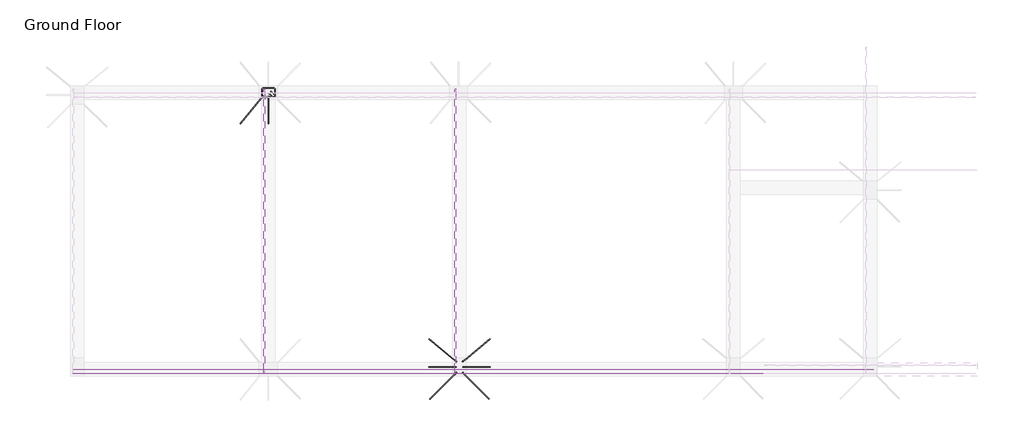
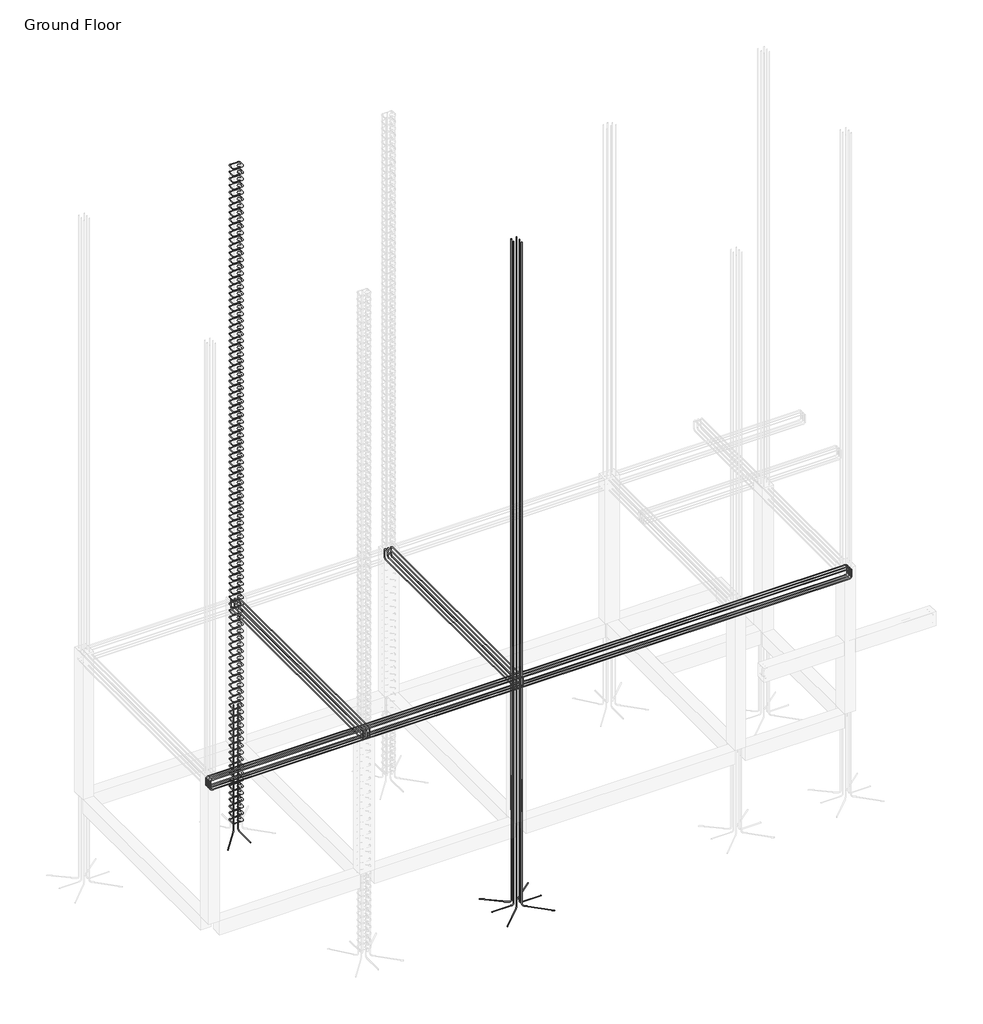
# One storey, part 3 of 5: 21 reinforcing bars.
"""IFC4 building model written with IfcOpenShell, lengths in millimetres."""

from ifc_helpers import new_model, si_unit, point, frame, origin, place, context, project, spatial, polyline, circle_curve, trimmed, segment, composite_curve, source, transform, mapped, element, save
from ifc_brep_helpers import swept_disk

model = new_model("IFC4")

# Units and contexts
model_context = context("Model", 3, world=origin())
ifc_project = project(units=[si_unit("LENGTHUNIT", "METRE", prefix="MILLI")], contexts=[model_context])

# Site, building, storey
site = spatial("IfcSite", under=ifc_project)
building = spatial("IfcBuilding", under=site)
storey = spatial("IfcBuildingStorey", under=building, Name="Ground Floor", Elevation=0.0)

# Reinforcing bars
placement = place(None, origin())
element("IfcReinforcingBar", 1, at=placement, inside=storey, context=model_context, shape_type="SolidModel", body=[
    swept_disk(composite_curve([segment(polyline([(-2783.7729913, 244.7072019, 877.2694454), (-2783.7729913, 244.7072019, -1868.0)]), True, "CONTINUOUS"), segment(trimmed(circle_curve(frame((-2751.2460793, 212.1802899, -1868.0), z_axis=(-0.7071067811865491, -0.707106781186546, 0.0), x_axis=(-32.52691199999981, 32.52691200000001, 0.0)), 46.0), [point((-2783.7729913, 244.7072019, -1868.0))], [point((-2751.2460793, 212.1802899, -1914.0))], True, "CARTESIAN"), True, "CONTINUOUS"), segment(polyline([(-2751.2460793, 212.1802899, -1914.0), (-2345.5428199, -193.5229695, -1914.0)]), True, "CONTINUOUS")], self_intersect=False), 6.0),
])
element("IfcReinforcingBar", 2, at=placement, inside=storey, context=model_context, shape_type="SolidModel", body=[
    swept_disk(composite_curve([segment(polyline([(-2892.5998971, 245.6611074, 884.8983833), (-2892.5998971, 245.6611074, -1868.0)]), True, "CONTINUOUS"), segment(trimmed(circle_curve(frame((-2925.126809, 213.1341954, -1868.0), z_axis=(-0.7071067811865491, 0.707106781186546, 0.0), x_axis=(32.52691189999996, 32.52691199999998, 0.0)), 46.0), [point((-2892.5998971, 245.6611074, -1868.0))], [point((-2925.126809, 213.1341954, -1914.0))], True, "CARTESIAN"), True, "CONTINUOUS"), segment(polyline([(-2925.126809, 213.1341954, -1914.0), (-3337.2563428, -198.9953384, -1914.0)]), True, "CONTINUOUS")], self_intersect=False), 6.0),
])
element("IfcReinforcingBar", 3, at=placement, inside=storey, context=model_context, shape_type="SolidModel", body=[
    swept_disk(composite_curve([segment(polyline([(-2785.0828277, 432.9867911, 871.8711989), (-2785.0828277, 432.9867911, -1868.0)]), True, "CONTINUOUS"), segment(trimmed(circle_curve(frame((-2749.5367573, 462.1839978, -1868.0), z_axis=(0.634721884628903, -0.7727406610067401, 0.0), x_axis=(-35.54607040000019, -29.19720669999998, 0.0)), 46.0), [point((-2785.0828277, 432.9867911, -1868.0))], [point((-2749.5367573, 462.1839978, -1914.0))], True, "CARTESIAN"), True, "CONTINUOUS"), segment(polyline([(-2749.5367573, 462.1839978, -1914.0), (-2327.2008173, 809.0867522, -1914.0)]), True, "CONTINUOUS")], self_intersect=False), 6.0),
])
element("IfcReinforcingBar", 4, at=placement, inside=storey, context=model_context, shape_type="SolidModel", body=[
    swept_disk(composite_curve([segment(polyline([(-2891.7839747, 432.7322479, 890.3940928), (-2891.7839747, 432.7322479, -1868.0)]), True, "CONTINUOUS"), segment(trimmed(circle_curve(frame((-2927.3300451, 461.9294546, -1868.0), z_axis=(0.634721884628903, 0.7727406610067401, 0.0), x_axis=(35.54607040000019, -29.19720669999998, 0.0)), 46.0), [point((-2891.7839747, 432.7322479, -1868.0))], [point((-2927.3300451, 461.9294546, -1914.0))], True, "CARTESIAN"), True, "CONTINUOUS"), segment(polyline([(-2927.3300451, 461.9294546, -1914.0), (-3351.4976875, 810.3367522, -1914.0)]), True, "CONTINUOUS")], self_intersect=False), 6.0),
])
element("IfcReinforcingBar", 5, at=placement, inside=storey, context=model_context, shape_type="SolidModel", body=[
    swept_disk(composite_curve([segment(polyline([(-2778.1117524, 339.6230123, 875.7528218), (-2778.1117524, 339.6230123, -1868.0)]), True, "CONTINUOUS"), segment(trimmed(circle_curve(frame((-2732.1117524, 339.6230123, -1868.0), z_axis=(0.0, -1.0, 0.0), x_axis=(-46.0, 0.0, 0.0)), 46.0), [point((-2778.1117524, 339.6230123, -1868.0))], [point((-2732.1117524, 339.6230123, -1914.0))], True, "CARTESIAN"), True, "CONTINUOUS"), segment(polyline([(-2732.1117524, 339.6230123, -1914.0), (-2321.1359391, 339.6230123, -1914.0)]), True, "CONTINUOUS")], self_intersect=False), 6.0),
])
element("IfcReinforcingBar", 6, at=placement, inside=storey, context=model_context, shape_type="SolidModel", body=[
    swept_disk(composite_curve([segment(polyline([(-2898.7117524, 339.6230123, 879.2840812), (-2898.7117524, 339.6230123, -1868.0)]), True, "CONTINUOUS"), segment(trimmed(circle_curve(frame((-2944.7117524, 339.6230123, -1868.0), z_axis=(0.0, 1.0, 0.0), x_axis=(46.0, 0.0, 0.0)), 46.0), [point((-2898.7117524, 339.6230123, -1868.0))], [point((-2944.7117524, 339.6230123, -1914.0))], True, "CARTESIAN"), True, "CONTINUOUS"), segment(polyline([(-2944.7117524, 339.6230123, -1914.0), (-3358.2222077, 339.6230123, -1914.0)]), True, "CONTINUOUS")], self_intersect=False), 6.0),
])
element("IfcReinforcingBar", 7, at=placement, inside=storey, context=model_context, shape_type="SolidModel", body=[
    swept_disk(composite_curve([segment(polyline([(-2782.2122575, 244.5339681, 12794.2305276), (-2782.2122575, 244.5339681, 171.0746196)]), True, "CONTINUOUS")], self_intersect=False), 6.0),
])
element("IfcReinforcingBar", 8, at=placement, inside=storey, context=model_context, shape_type="SolidModel", body=[
    swept_disk(composite_curve([segment(polyline([(-2778.1117524, 339.6230123, 888.7528218), (-2778.1117524, 339.6230123, 12792.7935546)]), True, "CONTINUOUS")], self_intersect=False), 6.0),
])
element("IfcReinforcingBar", 9, at=placement, inside=storey, context=model_context, shape_type="SolidModel", body=[
    swept_disk(composite_curve([segment(polyline([(-2782.2122575, 433.132958, 12790.6127039), (-2782.2122575, 433.132958, 154.6015232)]), True, "CONTINUOUS")], self_intersect=False), 6.0),
])
element("IfcReinforcingBar", 10, at=placement, inside=storey, context=model_context, shape_type="SolidModel", body=[
    swept_disk(composite_curve([segment(polyline([(-2894.6112474, 244.5339681, 12794.2305276), (-2894.6112474, 244.5339681, 159.2991411)]), True, "CONTINUOUS")], self_intersect=False), 6.0),
])
element("IfcReinforcingBar", 11, at=placement, inside=storey, context=model_context, shape_type="SolidModel", body=[
    swept_disk(composite_curve([segment(polyline([(-2898.7117524, 339.6230123, 892.2840812), (-2898.7117524, 339.6230123, 12792.7935546)]), True, "CONTINUOUS")], self_intersect=False), 6.0),
])
element("IfcReinforcingBar", 12, at=placement, inside=storey, context=model_context, shape_type="SolidModel", body=[
    swept_disk(composite_curve([segment(polyline([(-2894.6112474, 433.132958, 12790.6127039), (-2894.6112474, 433.132958, 134.6074908)]), True, "CONTINUOUS")], self_intersect=False), 6.0),
])
element("IfcReinforcingBar", 13, at=placement, inside=storey, context=model_context, shape_type="SolidModel", body=[
    swept_disk(composite_curve([segment(polyline([(-6145.4105373, 4895.5612408, 890.3940928), (-6145.4105373, 4895.5612408, -1868.0)]), True, "CONTINUOUS"), segment(trimmed(circle_curve(frame((-6174.607744, 4860.0151704, -1868.0), z_axis=(-0.772740661006739, 0.6347218846289044, 0.0), x_axis=(29.197206699999697, 35.546070399999735, 0.0)), 46.0), [point((-6145.4105373, 4895.5612408, -1868.0))], [point((-6174.607744, 4860.0151704, -1914.0))], True, "CARTESIAN"), True, "CONTINUOUS"), segment(polyline([(-6174.607744, 4860.0151704, -1914.0), (-6523.0150416, 4435.8475279, -1914.0)]), True, "CONTINUOUS")], self_intersect=False), 6.0),
])
element("IfcReinforcingBar", 14, at=placement, inside=storey, context=model_context, shape_type="SolidModel", body=[
    swept_disk(composite_curve([segment(polyline([(-6052.3013017, 4888.6334631, 879.2840812), (-6052.3013017, 4888.6334631, -1868.0)]), True, "CONTINUOUS"), segment(trimmed(circle_curve(frame((-6052.3013017, 4842.6334631, -1868.0), z_axis=(-1.0, 0.0, 0.0), x_axis=(0.0, 46.0, 0.0)), 46.0), [point((-6052.3013017, 4888.6334631, -1868.0))], [point((-6052.3013017, 4842.6334631, -1914.0))], True, "CARTESIAN"), True, "CONTINUOUS"), segment(polyline([(-6052.3013017, 4842.6334631, -1914.0), (-6052.3013017, 4429.1230078, -1914.0)]), True, "CONTINUOUS")], self_intersect=False), 6.0),
])
reinforcing_bar_shape = source(origin(), model_context, "Body", "SolidModel", [
    swept_disk(composite_curve([segment(polyline([(-6041.6771046, 4943.2576897, -1724.0), (-5984.0823152, 4885.6629003, -1724.0)]), True, "CONTINUOUS"), segment(trimmed(circle_curve(frame((-5967.1117524, 4902.6334631, -1724.0), z_axis=(0.0, 0.0, 1.0), x_axis=(-16.970562800000152, -16.970562800000152, 0.0)), 24.0), [point((-5984.0823152, 4885.6629003, -1724.0))], [point((-5943.1117524, 4902.6334631, -1724.0))], True, "CARTESIAN"), True, "CONTINUOUS"), segment(polyline([(-5943.1117524, 4902.6334631, -1724.0), (-5943.1117524, 5010.2334631, -1724.0)]), True, "CONTINUOUS"), segment(trimmed(circle_curve(frame((-5967.1117524, 5010.2334631, -1724.0), z_axis=(0.0, 0.0, 1.0), x_axis=(24.0, 0.0, 0.0)), 24.0), [point((-5943.1117524, 5010.2334631, -1724.0))], [point((-5967.1117524, 5034.2334631, -1724.0))], True, "CARTESIAN"), True, "CONTINUOUS"), segment(polyline([(-5967.1117524, 5034.2334631, -1724.0), (-6135.9117524, 5034.2334631, -1724.0)]), True, "CONTINUOUS"), segment(trimmed(circle_curve(frame((-6135.9117524, 5010.2651209, -1725.2323055), z_axis=(0.0, -0.05134606277295722, 0.9986809209340667), x_axis=(0.0, 23.968342200000734, 1.2323054999999385)), 24.0), [point((-6135.9117524, 5034.2334631, -1724.0))], [point((-6159.9117524, 5010.2651209, -1725.2323055))], True, "CARTESIAN"), True, "CONTINUOUS"), segment(polyline([(-6159.9117524, 5010.2651209, -1725.2323055), (-6159.9117524, 4902.6018052, -1730.7676945)]), True, "CONTINUOUS"), segment(trimmed(circle_curve(frame((-6135.9117524, 4902.6018052, -1730.7676945), z_axis=(0.0, -0.05134606277295722, 0.9986809209340667), x_axis=(-24.0, 0.0, 0.0)), 24.0), [point((-6159.9117524, 4902.6018052, -1730.7676945))], [point((-6135.9117524, 4878.6334631, -1732.0))], True, "CARTESIAN"), True, "CONTINUOUS"), segment(polyline([(-6135.9117524, 4878.6334631, -1732.0), (-5967.1117524, 4878.6334631, -1732.0)]), True, "CONTINUOUS"), segment(trimmed(circle_curve(frame((-5967.1117524, 4902.6334631, -1732.0), z_axis=(0.0, 0.0, 1.0), x_axis=(0.0, -24.0, 0.0)), 24.0), [point((-5967.1117524, 4878.6334631, -1732.0))], [point((-5950.1411897, 4919.6040258, -1732.0))], True, "CARTESIAN"), True, "CONTINUOUS"), segment(polyline([(-5950.1411897, 4919.6040258, -1732.0), (-6007.7359791, 4977.1988152, -1732.0)]), True, "CONTINUOUS")], self_intersect=False), 4.0),
])
element("IfcReinforcingBar", 15, at=placement, inside=storey, context=model_context, shape_type="MappedRepresentation", body=[
    mapped(reinforcing_bar_shape, transform((0.0, 0.0, 0.0), x_axis=(1.0, 0.0, 0.0), y_axis=(0.0, 1.0, 0.0), z_axis=(0.0, 0.0, 1.0))),
    mapped(reinforcing_bar_shape, transform((0.0, 0.0, 149.5904239), x_axis=(1.0, 0.0, 0.0), y_axis=(0.0, 1.0, 0.0), z_axis=(0.0, 0.0, 1.0))),
    mapped(reinforcing_bar_shape, transform((0.0, 0.0, 299.1808479), x_axis=(1.0, 0.0, 0.0), y_axis=(0.0, 1.0, 0.0), z_axis=(0.0, 0.0, 1.0))),
    mapped(reinforcing_bar_shape, transform((0.0, 0.0, 448.7712718), x_axis=(1.0, 0.0, 0.0), y_axis=(0.0, 1.0, 0.0), z_axis=(0.0, 0.0, 1.0))),
    mapped(reinforcing_bar_shape, transform((0.0, 0.0, 598.3616957), x_axis=(1.0, 0.0, 0.0), y_axis=(0.0, 1.0, 0.0), z_axis=(0.0, 0.0, 1.0))),
    mapped(reinforcing_bar_shape, transform((0.0, 0.0, 747.9521197), x_axis=(1.0, 0.0, 0.0), y_axis=(0.0, 1.0, 0.0), z_axis=(0.0, 0.0, 1.0))),
    mapped(reinforcing_bar_shape, transform((0.0, 0.0, 897.5425436), x_axis=(1.0, 0.0, 0.0), y_axis=(0.0, 1.0, 0.0), z_axis=(0.0, 0.0, 1.0))),
    mapped(reinforcing_bar_shape, transform((0.0, 0.0, 1047.1329675), x_axis=(1.0, 0.0, 0.0), y_axis=(0.0, 1.0, 0.0), z_axis=(0.0, 0.0, 1.0))),
    mapped(reinforcing_bar_shape, transform((0.0, 0.0, 1196.7233914), x_axis=(1.0, 0.0, 0.0), y_axis=(0.0, 1.0, 0.0), z_axis=(0.0, 0.0, 1.0))),
    mapped(reinforcing_bar_shape, transform((0.0, 0.0, 1346.3138154), x_axis=(1.0, 0.0, 0.0), y_axis=(0.0, 1.0, 0.0), z_axis=(0.0, 0.0, 1.0))),
    mapped(reinforcing_bar_shape, transform((0.0, 0.0, 1495.9042393), x_axis=(1.0, 0.0, 0.0), y_axis=(0.0, 1.0, 0.0), z_axis=(0.0, 0.0, 1.0))),
    mapped(reinforcing_bar_shape, transform((0.0, 0.0, 1645.4946632), x_axis=(1.0, 0.0, 0.0), y_axis=(0.0, 1.0, 0.0), z_axis=(0.0, 0.0, 1.0))),
    mapped(reinforcing_bar_shape, transform((0.0, 0.0, 1795.0850872), x_axis=(1.0, 0.0, 0.0), y_axis=(0.0, 1.0, 0.0), z_axis=(0.0, 0.0, 1.0))),
    mapped(reinforcing_bar_shape, transform((0.0, 0.0, 1944.6755111), x_axis=(1.0, 0.0, 0.0), y_axis=(0.0, 1.0, 0.0), z_axis=(0.0, 0.0, 1.0))),
    mapped(reinforcing_bar_shape, transform((0.0, 0.0, 2094.265935), x_axis=(1.0, 0.0, 0.0), y_axis=(0.0, 1.0, 0.0), z_axis=(0.0, 0.0, 1.0))),
    mapped(reinforcing_bar_shape, transform((0.0, 0.0, 2243.856359), x_axis=(1.0, 0.0, 0.0), y_axis=(0.0, 1.0, 0.0), z_axis=(0.0, 0.0, 1.0))),
    mapped(reinforcing_bar_shape, transform((0.0, 0.0, 2393.4467829), x_axis=(1.0, 0.0, 0.0), y_axis=(0.0, 1.0, 0.0), z_axis=(0.0, 0.0, 1.0))),
    mapped(reinforcing_bar_shape, transform((0.0, 0.0, 2543.0372068), x_axis=(1.0, 0.0, 0.0), y_axis=(0.0, 1.0, 0.0), z_axis=(0.0, 0.0, 1.0))),
    mapped(reinforcing_bar_shape, transform((0.0, 0.0, 2692.6276307), x_axis=(1.0, 0.0, 0.0), y_axis=(0.0, 1.0, 0.0), z_axis=(0.0, 0.0, 1.0))),
    mapped(reinforcing_bar_shape, transform((0.0, 0.0, 2842.2180547), x_axis=(1.0, 0.0, 0.0), y_axis=(0.0, 1.0, 0.0), z_axis=(0.0, 0.0, 1.0))),
    mapped(reinforcing_bar_shape, transform((0.0, 0.0, 2991.8084786), x_axis=(1.0, 0.0, 0.0), y_axis=(0.0, 1.0, 0.0), z_axis=(0.0, 0.0, 1.0))),
    mapped(reinforcing_bar_shape, transform((0.0, 0.0, 3141.3989025), x_axis=(1.0, 0.0, 0.0), y_axis=(0.0, 1.0, 0.0), z_axis=(0.0, 0.0, 1.0))),
    mapped(reinforcing_bar_shape, transform((0.0, 0.0, 3290.9893265), x_axis=(1.0, 0.0, 0.0), y_axis=(0.0, 1.0, 0.0), z_axis=(0.0, 0.0, 1.0))),
    mapped(reinforcing_bar_shape, transform((0.0, 0.0, 3440.5797504), x_axis=(1.0, 0.0, 0.0), y_axis=(0.0, 1.0, 0.0), z_axis=(0.0, 0.0, 1.0))),
    mapped(reinforcing_bar_shape, transform((0.0, 0.0, 3590.1701743), x_axis=(1.0, 0.0, 0.0), y_axis=(0.0, 1.0, 0.0), z_axis=(0.0, 0.0, 1.0))),
    mapped(reinforcing_bar_shape, transform((0.0, 0.0, 3739.7605983), x_axis=(1.0, 0.0, 0.0), y_axis=(0.0, 1.0, 0.0), z_axis=(0.0, 0.0, 1.0))),
    mapped(reinforcing_bar_shape, transform((0.0, 0.0, 3889.3510222), x_axis=(1.0, 0.0, 0.0), y_axis=(0.0, 1.0, 0.0), z_axis=(0.0, 0.0, 1.0))),
    mapped(reinforcing_bar_shape, transform((0.0, 0.0, 4038.9414461), x_axis=(1.0, 0.0, 0.0), y_axis=(0.0, 1.0, 0.0), z_axis=(0.0, 0.0, 1.0))),
    mapped(reinforcing_bar_shape, transform((0.0, 0.0, 4188.53187), x_axis=(1.0, 0.0, 0.0), y_axis=(0.0, 1.0, 0.0), z_axis=(0.0, 0.0, 1.0))),
    mapped(reinforcing_bar_shape, transform((0.0, 0.0, 4338.122294), x_axis=(1.0, 0.0, 0.0), y_axis=(0.0, 1.0, 0.0), z_axis=(0.0, 0.0, 1.0))),
    mapped(reinforcing_bar_shape, transform((0.0, 0.0, 4487.7127179), x_axis=(1.0, 0.0, 0.0), y_axis=(0.0, 1.0, 0.0), z_axis=(0.0, 0.0, 1.0))),
    mapped(reinforcing_bar_shape, transform((0.0, 0.0, 4637.3031418), x_axis=(1.0, 0.0, 0.0), y_axis=(0.0, 1.0, 0.0), z_axis=(0.0, 0.0, 1.0))),
    mapped(reinforcing_bar_shape, transform((0.0, 0.0, 4786.8935658), x_axis=(1.0, 0.0, 0.0), y_axis=(0.0, 1.0, 0.0), z_axis=(0.0, 0.0, 1.0))),
    mapped(reinforcing_bar_shape, transform((0.0, 0.0, 4936.4839897), x_axis=(1.0, 0.0, 0.0), y_axis=(0.0, 1.0, 0.0), z_axis=(0.0, 0.0, 1.0))),
    mapped(reinforcing_bar_shape, transform((0.0, 0.0, 5086.0744136), x_axis=(1.0, 0.0, 0.0), y_axis=(0.0, 1.0, 0.0), z_axis=(0.0, 0.0, 1.0))),
    mapped(reinforcing_bar_shape, transform((0.0, 0.0, 5235.6648376), x_axis=(1.0, 0.0, 0.0), y_axis=(0.0, 1.0, 0.0), z_axis=(0.0, 0.0, 1.0))),
    mapped(reinforcing_bar_shape, transform((0.0, 0.0, 5385.2552615), x_axis=(1.0, 0.0, 0.0), y_axis=(0.0, 1.0, 0.0), z_axis=(0.0, 0.0, 1.0))),
    mapped(reinforcing_bar_shape, transform((0.0, 0.0, 5534.8456854), x_axis=(1.0, 0.0, 0.0), y_axis=(0.0, 1.0, 0.0), z_axis=(0.0, 0.0, 1.0))),
    mapped(reinforcing_bar_shape, transform((0.0, 0.0, 5684.4361094), x_axis=(1.0, 0.0, 0.0), y_axis=(0.0, 1.0, 0.0), z_axis=(0.0, 0.0, 1.0))),
    mapped(reinforcing_bar_shape, transform((0.0, 0.0, 5834.0265333), x_axis=(1.0, 0.0, 0.0), y_axis=(0.0, 1.0, 0.0), z_axis=(0.0, 0.0, 1.0))),
    mapped(reinforcing_bar_shape, transform((0.0, 0.0, 5983.6169572), x_axis=(1.0, 0.0, 0.0), y_axis=(0.0, 1.0, 0.0), z_axis=(0.0, 0.0, 1.0))),
    mapped(reinforcing_bar_shape, transform((0.0, 0.0, 6133.2073811), x_axis=(1.0, 0.0, 0.0), y_axis=(0.0, 1.0, 0.0), z_axis=(0.0, 0.0, 1.0))),
    mapped(reinforcing_bar_shape, transform((0.0, 0.0, 6282.7978051), x_axis=(1.0, 0.0, 0.0), y_axis=(0.0, 1.0, 0.0), z_axis=(0.0, 0.0, 1.0))),
    mapped(reinforcing_bar_shape, transform((0.0, 0.0, 6432.388229), x_axis=(1.0, 0.0, 0.0), y_axis=(0.0, 1.0, 0.0), z_axis=(0.0, 0.0, 1.0))),
    mapped(reinforcing_bar_shape, transform((0.0, 0.0, 6581.9786529), x_axis=(1.0, 0.0, 0.0), y_axis=(0.0, 1.0, 0.0), z_axis=(0.0, 0.0, 1.0))),
    mapped(reinforcing_bar_shape, transform((0.0, 0.0, 6731.5690769), x_axis=(1.0, 0.0, 0.0), y_axis=(0.0, 1.0, 0.0), z_axis=(0.0, 0.0, 1.0))),
    mapped(reinforcing_bar_shape, transform((0.0, 0.0, 6881.1595008), x_axis=(1.0, 0.0, 0.0), y_axis=(0.0, 1.0, 0.0), z_axis=(0.0, 0.0, 1.0))),
    mapped(reinforcing_bar_shape, transform((0.0, 0.0, 7030.7499247), x_axis=(1.0, 0.0, 0.0), y_axis=(0.0, 1.0, 0.0), z_axis=(0.0, 0.0, 1.0))),
    mapped(reinforcing_bar_shape, transform((0.0, 0.0, 7180.3403487), x_axis=(1.0, 0.0, 0.0), y_axis=(0.0, 1.0, 0.0), z_axis=(0.0, 0.0, 1.0))),
    mapped(reinforcing_bar_shape, transform((0.0, 0.0, 7329.9307726), x_axis=(1.0, 0.0, 0.0), y_axis=(0.0, 1.0, 0.0), z_axis=(0.0, 0.0, 1.0))),
    mapped(reinforcing_bar_shape, transform((0.0, 0.0, 7479.5211965), x_axis=(1.0, 0.0, 0.0), y_axis=(0.0, 1.0, 0.0), z_axis=(0.0, 0.0, 1.0))),
    mapped(reinforcing_bar_shape, transform((0.0, 0.0, 7629.1116204), x_axis=(1.0, 0.0, 0.0), y_axis=(0.0, 1.0, 0.0), z_axis=(0.0, 0.0, 1.0))),
    mapped(reinforcing_bar_shape, transform((0.0, 0.0, 7778.7020444), x_axis=(1.0, 0.0, 0.0), y_axis=(0.0, 1.0, 0.0), z_axis=(0.0, 0.0, 1.0))),
    mapped(reinforcing_bar_shape, transform((0.0, 0.0, 7928.2924683), x_axis=(1.0, 0.0, 0.0), y_axis=(0.0, 1.0, 0.0), z_axis=(0.0, 0.0, 1.0))),
    mapped(reinforcing_bar_shape, transform((0.0, 0.0, 8077.8828922), x_axis=(1.0, 0.0, 0.0), y_axis=(0.0, 1.0, 0.0), z_axis=(0.0, 0.0, 1.0))),
    mapped(reinforcing_bar_shape, transform((0.0, 0.0, 8227.4733162), x_axis=(1.0, 0.0, 0.0), y_axis=(0.0, 1.0, 0.0), z_axis=(0.0, 0.0, 1.0))),
    mapped(reinforcing_bar_shape, transform((0.0, 0.0, 8377.0637401), x_axis=(1.0, 0.0, 0.0), y_axis=(0.0, 1.0, 0.0), z_axis=(0.0, 0.0, 1.0))),
    mapped(reinforcing_bar_shape, transform((0.0, 0.0, 8526.654164), x_axis=(1.0, 0.0, 0.0), y_axis=(0.0, 1.0, 0.0), z_axis=(0.0, 0.0, 1.0))),
    mapped(reinforcing_bar_shape, transform((0.0, 0.0, 8676.244588), x_axis=(1.0, 0.0, 0.0), y_axis=(0.0, 1.0, 0.0), z_axis=(0.0, 0.0, 1.0))),
    mapped(reinforcing_bar_shape, transform((0.0, 0.0, 8825.8350119), x_axis=(1.0, 0.0, 0.0), y_axis=(0.0, 1.0, 0.0), z_axis=(0.0, 0.0, 1.0))),
    mapped(reinforcing_bar_shape, transform((0.0, 0.0, 8975.4254358), x_axis=(1.0, 0.0, 0.0), y_axis=(0.0, 1.0, 0.0), z_axis=(0.0, 0.0, 1.0))),
    mapped(reinforcing_bar_shape, transform((0.0, 0.0, 9125.0158597), x_axis=(1.0, 0.0, 0.0), y_axis=(0.0, 1.0, 0.0), z_axis=(0.0, 0.0, 1.0))),
    mapped(reinforcing_bar_shape, transform((0.0, 0.0, 9274.6062837), x_axis=(1.0, 0.0, 0.0), y_axis=(0.0, 1.0, 0.0), z_axis=(0.0, 0.0, 1.0))),
    mapped(reinforcing_bar_shape, transform((0.0, 0.0, 9424.1967076), x_axis=(1.0, 0.0, 0.0), y_axis=(0.0, 1.0, 0.0), z_axis=(0.0, 0.0, 1.0))),
    mapped(reinforcing_bar_shape, transform((0.0, 0.0, 9573.7871315), x_axis=(1.0, 0.0, 0.0), y_axis=(0.0, 1.0, 0.0), z_axis=(0.0, 0.0, 1.0))),
    mapped(reinforcing_bar_shape, transform((0.0, 0.0, 9723.3775555), x_axis=(1.0, 0.0, 0.0), y_axis=(0.0, 1.0, 0.0), z_axis=(0.0, 0.0, 1.0))),
    mapped(reinforcing_bar_shape, transform((0.0, 0.0, 9872.9679794), x_axis=(1.0, 0.0, 0.0), y_axis=(0.0, 1.0, 0.0), z_axis=(0.0, 0.0, 1.0))),
    mapped(reinforcing_bar_shape, transform((0.0, 0.0, 10022.5584033), x_axis=(1.0, 0.0, 0.0), y_axis=(0.0, 1.0, 0.0), z_axis=(0.0, 0.0, 1.0))),
    mapped(reinforcing_bar_shape, transform((0.0, 0.0, 10172.1488273), x_axis=(1.0, 0.0, 0.0), y_axis=(0.0, 1.0, 0.0), z_axis=(0.0, 0.0, 1.0))),
    mapped(reinforcing_bar_shape, transform((0.0, 0.0, 10321.7392512), x_axis=(1.0, 0.0, 0.0), y_axis=(0.0, 1.0, 0.0), z_axis=(0.0, 0.0, 1.0))),
    mapped(reinforcing_bar_shape, transform((0.0, 0.0, 10471.3296751), x_axis=(1.0, 0.0, 0.0), y_axis=(0.0, 1.0, 0.0), z_axis=(0.0, 0.0, 1.0))),
    mapped(reinforcing_bar_shape, transform((0.0, 0.0, 10620.9200991), x_axis=(1.0, 0.0, 0.0), y_axis=(0.0, 1.0, 0.0), z_axis=(0.0, 0.0, 1.0))),
    mapped(reinforcing_bar_shape, transform((0.0, 0.0, 10770.510523), x_axis=(1.0, 0.0, 0.0), y_axis=(0.0, 1.0, 0.0), z_axis=(0.0, 0.0, 1.0))),
    mapped(reinforcing_bar_shape, transform((0.0, 0.0, 10920.1009469), x_axis=(1.0, 0.0, 0.0), y_axis=(0.0, 1.0, 0.0), z_axis=(0.0, 0.0, 1.0))),
    mapped(reinforcing_bar_shape, transform((0.0, 0.0, 11069.6913708), x_axis=(1.0, 0.0, 0.0), y_axis=(0.0, 1.0, 0.0), z_axis=(0.0, 0.0, 1.0))),
    mapped(reinforcing_bar_shape, transform((0.0, 0.0, 11219.2817948), x_axis=(1.0, 0.0, 0.0), y_axis=(0.0, 1.0, 0.0), z_axis=(0.0, 0.0, 1.0))),
    mapped(reinforcing_bar_shape, transform((0.0, 0.0, 11368.8722187), x_axis=(1.0, 0.0, 0.0), y_axis=(0.0, 1.0, 0.0), z_axis=(0.0, 0.0, 1.0))),
    mapped(reinforcing_bar_shape, transform((0.0, 0.0, 11518.4626426), x_axis=(1.0, 0.0, 0.0), y_axis=(0.0, 1.0, 0.0), z_axis=(0.0, 0.0, 1.0))),
    mapped(reinforcing_bar_shape, transform((0.0, 0.0, 11668.0530666), x_axis=(1.0, 0.0, 0.0), y_axis=(0.0, 1.0, 0.0), z_axis=(0.0, 0.0, 1.0))),
    mapped(reinforcing_bar_shape, transform((0.0, 0.0, 11817.6434905), x_axis=(1.0, 0.0, 0.0), y_axis=(0.0, 1.0, 0.0), z_axis=(0.0, 0.0, 1.0))),
    mapped(reinforcing_bar_shape, transform((0.0, 0.0, 11967.2339144), x_axis=(1.0, 0.0, 0.0), y_axis=(0.0, 1.0, 0.0), z_axis=(0.0, 0.0, 1.0))),
    mapped(reinforcing_bar_shape, transform((0.0, 0.0, 12116.8243384), x_axis=(1.0, 0.0, 0.0), y_axis=(0.0, 1.0, 0.0), z_axis=(0.0, 0.0, 1.0))),
    mapped(reinforcing_bar_shape, transform((0.0, 0.0, 12266.4147623), x_axis=(1.0, 0.0, 0.0), y_axis=(0.0, 1.0, 0.0), z_axis=(0.0, 0.0, 1.0))),
    mapped(reinforcing_bar_shape, transform((0.0, 0.0, 12416.0051862), x_axis=(1.0, 0.0, 0.0), y_axis=(0.0, 1.0, 0.0), z_axis=(0.0, 0.0, 1.0))),
    mapped(reinforcing_bar_shape, transform((0.0, 0.0, 12565.5956101), x_axis=(1.0, 0.0, 0.0), y_axis=(0.0, 1.0, 0.0), z_axis=(0.0, 0.0, 1.0))),
    mapped(reinforcing_bar_shape, transform((0.0, 0.0, 12715.1860341), x_axis=(1.0, 0.0, 0.0), y_axis=(0.0, 1.0, 0.0), z_axis=(0.0, 0.0, 1.0))),
    mapped(reinforcing_bar_shape, transform((0.0, 0.0, 12864.776458), x_axis=(1.0, 0.0, 0.0), y_axis=(0.0, 1.0, 0.0), z_axis=(0.0, 0.0, 1.0))),
    mapped(reinforcing_bar_shape, transform((0.0, 0.0, 13014.3668819), x_axis=(1.0, 0.0, 0.0), y_axis=(0.0, 1.0, 0.0), z_axis=(0.0, 0.0, 1.0))),
    mapped(reinforcing_bar_shape, transform((0.0, 0.0, 13163.9573059), x_axis=(1.0, 0.0, 0.0), y_axis=(0.0, 1.0, 0.0), z_axis=(0.0, 0.0, 1.0))),
    mapped(reinforcing_bar_shape, transform((0.0, 0.0, 13313.5477298), x_axis=(1.0, 0.0, 0.0), y_axis=(0.0, 1.0, 0.0), z_axis=(0.0, 0.0, 1.0))),
    mapped(reinforcing_bar_shape, transform((0.0, 0.0, 13463.1381537), x_axis=(1.0, 0.0, 0.0), y_axis=(0.0, 1.0, 0.0), z_axis=(0.0, 0.0, 1.0))),
    mapped(reinforcing_bar_shape, transform((0.0, 0.0, 13612.7285777), x_axis=(1.0, 0.0, 0.0), y_axis=(0.0, 1.0, 0.0), z_axis=(0.0, 0.0, 1.0))),
    mapped(reinforcing_bar_shape, transform((0.0, 0.0, 13762.3190016), x_axis=(1.0, 0.0, 0.0), y_axis=(0.0, 1.0, 0.0), z_axis=(0.0, 0.0, 1.0))),
    mapped(reinforcing_bar_shape, transform((0.0, 0.0, 13911.9094255), x_axis=(1.0, 0.0, 0.0), y_axis=(0.0, 1.0, 0.0), z_axis=(0.0, 0.0, 1.0))),
    mapped(reinforcing_bar_shape, transform((0.0, 0.0, 14061.4998494), x_axis=(1.0, 0.0, 0.0), y_axis=(0.0, 1.0, 0.0), z_axis=(0.0, 0.0, 1.0))),
    mapped(reinforcing_bar_shape, transform((0.0, 0.0, 14211.0902734), x_axis=(1.0, 0.0, 0.0), y_axis=(0.0, 1.0, 0.0), z_axis=(0.0, 0.0, 1.0))),
    mapped(reinforcing_bar_shape, transform((0.0, 0.0, 14360.6806973), x_axis=(1.0, 0.0, 0.0), y_axis=(0.0, 1.0, 0.0), z_axis=(0.0, 0.0, 1.0))),
    mapped(reinforcing_bar_shape, transform((0.0, 0.0, 14510.2711212), x_axis=(1.0, 0.0, 0.0), y_axis=(0.0, 1.0, 0.0), z_axis=(0.0, 0.0, 1.0))),
])
reinforcing_bar_2_shape = source(origin(), model_context, "Body", "SolidModel", [
    swept_disk(composite_curve([segment(polyline([(-2909.6112474, 5017.2334631, 2963.2994949), (-2909.6112474, 5017.2334631, 3111.2994949)]), True, "CONTINUOUS"), segment(trimmed(circle_curve(frame((-2909.6112474, 4971.2334631, 3111.2994949), z_axis=(1.0, 0.0, 0.0), x_axis=(0.0, 46.0, 0.0)), 46.0), [point((-2909.6112474, 5017.2334631, 3111.2994949))], [point((-2909.6112474, 4971.2334631, 3157.2994949))], True, "CARTESIAN"), True, "CONTINUOUS"), segment(polyline([(-2909.6112474, 4971.2334631, 3157.2994949), (-2909.6112474, 278.4334631, 3157.2994949)]), True, "CONTINUOUS"), segment(trimmed(circle_curve(frame((-2909.6112474, 278.4334631, 3111.2994949), z_axis=(1.0, 0.0, 0.0), x_axis=(0.0, 0.0, 46.0)), 46.0), [point((-2909.6112474, 278.4334631, 3157.2994949))], [point((-2909.6112474, 232.4334631, 3111.2994949))], True, "CARTESIAN"), True, "CONTINUOUS"), segment(polyline([(-2909.6112474, 232.4334631, 3111.2994949), (-2909.6112474, 232.4334631, 2963.2994949)]), True, "CONTINUOUS")], self_intersect=False), 6.0),
])
element("IfcReinforcingBar", 16, at=placement, inside=storey, context=model_context, shape_type="MappedRepresentation", body=[
    mapped(reinforcing_bar_2_shape, transform((0.0, 0.0, 0.0), x_axis=(1.0, 0.0, 0.0), y_axis=(0.0, 1.0, 0.0), z_axis=(0.0, 0.0, 1.0))),
    mapped(reinforcing_bar_2_shape, transform((71.1994949, 0.0, 0.0), x_axis=(1.0, 0.0, 0.0), y_axis=(0.0, 1.0, 0.0), z_axis=(0.0, 0.0, 1.0))),
    mapped(reinforcing_bar_2_shape, transform((142.3989899, 0.0, 0.0), x_axis=(1.0, 0.0, 0.0), y_axis=(0.0, 1.0, 0.0), z_axis=(0.0, 0.0, 1.0))),
])
reinforcing_bar_3_shape = source(origin(), model_context, "Body", "SolidModel", [
    swept_disk(composite_curve([segment(polyline([(-2909.6112474, 5017.2334631, 3132.7005051), (-2909.6112474, 5017.2334631, 2984.7005051)]), True, "CONTINUOUS"), segment(trimmed(circle_curve(frame((-2909.6112474, 4971.2334631, 2984.7005051), z_axis=(-1.0, 0.0, 0.0), x_axis=(0.0, 46.0, 0.0)), 46.0), [point((-2909.6112474, 5017.2334631, 2984.7005051))], [point((-2909.6112474, 4971.2334631, 2938.7005051))], True, "CARTESIAN"), True, "CONTINUOUS"), segment(polyline([(-2909.6112474, 4971.2334631, 2938.7005051), (-2909.6112474, 278.4334631, 2938.7005051)]), True, "CONTINUOUS"), segment(trimmed(circle_curve(frame((-2909.6112474, 278.4334631, 2984.7005051), z_axis=(-1.0, 0.0, 0.0), x_axis=(0.0, 0.0, -46.0)), 46.0), [point((-2909.6112474, 278.4334631, 2938.7005051))], [point((-2909.6112474, 232.4334631, 2984.7005051))], True, "CARTESIAN"), True, "CONTINUOUS"), segment(polyline([(-2909.6112474, 232.4334631, 2984.7005051), (-2909.6112474, 232.4334631, 3132.7005051)]), True, "CONTINUOUS")], self_intersect=False), 6.0),
])
element("IfcReinforcingBar", 17, at=placement, inside=storey, context=model_context, shape_type="MappedRepresentation", body=[
    mapped(reinforcing_bar_3_shape, transform((0.0, 0.0, 0.0), x_axis=(1.0, 0.0, 0.0), y_axis=(0.0, 1.0, 0.0), z_axis=(0.0, 0.0, 1.0))),
    mapped(reinforcing_bar_3_shape, transform((71.1994949, 0.0, 0.0), x_axis=(1.0, 0.0, 0.0), y_axis=(0.0, 1.0, 0.0), z_axis=(0.0, 0.0, 1.0))),
    mapped(reinforcing_bar_3_shape, transform((142.3989899, 0.0, 0.0), x_axis=(1.0, 0.0, 0.0), y_axis=(0.0, 1.0, 0.0), z_axis=(0.0, 0.0, 1.0))),
])
reinforcing_bar_4_shape = source(origin(), model_context, "Body", "SolidModel", [
    swept_disk(composite_curve([segment(polyline([(-6122.7112474, 5017.2334631, 2963.2994949), (-6122.7112474, 5017.2334631, 3111.2994949)]), True, "CONTINUOUS"), segment(trimmed(circle_curve(frame((-6122.7112474, 4971.2334631, 3111.2994949), z_axis=(1.0, 0.0, 0.0), x_axis=(0.0, 46.0, 0.0)), 46.0), [point((-6122.7112474, 5017.2334631, 3111.2994949))], [point((-6122.7112474, 4971.2334631, 3157.2994949))], True, "CARTESIAN"), True, "CONTINUOUS"), segment(polyline([(-6122.7112474, 4971.2334631, 3157.2994949), (-6122.7112474, 278.4334631, 3157.2994949)]), True, "CONTINUOUS"), segment(trimmed(circle_curve(frame((-6122.7112474, 278.4334631, 3111.2994949), z_axis=(1.0, 0.0, 0.0), x_axis=(0.0, 0.0, 46.0)), 46.0), [point((-6122.7112474, 278.4334631, 3157.2994949))], [point((-6122.7112474, 232.4334631, 3111.2994949))], True, "CARTESIAN"), True, "CONTINUOUS"), segment(polyline([(-6122.7112474, 232.4334631, 3111.2994949), (-6122.7112474, 232.4334631, 2963.2994949)]), True, "CONTINUOUS")], self_intersect=False), 6.0),
])
element("IfcReinforcingBar", 18, at=placement, inside=storey, context=model_context, shape_type="MappedRepresentation", body=[
    mapped(reinforcing_bar_4_shape, transform((0.0, 0.0, 0.0), x_axis=(1.0, 0.0, 0.0), y_axis=(0.0, 1.0, 0.0), z_axis=(0.0, 0.0, 1.0))),
    mapped(reinforcing_bar_4_shape, transform((71.1994949, 0.0, 0.0), x_axis=(1.0, 0.0, 0.0), y_axis=(0.0, 1.0, 0.0), z_axis=(0.0, 0.0, 1.0))),
    mapped(reinforcing_bar_4_shape, transform((142.3989899, 0.0, 0.0), x_axis=(1.0, 0.0, 0.0), y_axis=(0.0, 1.0, 0.0), z_axis=(0.0, 0.0, 1.0))),
])
reinforcing_bar_5_shape = source(origin(), model_context, "Body", "SolidModel", [
    swept_disk(composite_curve([segment(polyline([(-6122.7112474, 5017.2334631, 3132.7005051), (-6122.7112474, 5017.2334631, 2984.7005051)]), True, "CONTINUOUS"), segment(trimmed(circle_curve(frame((-6122.7112474, 4971.2334631, 2984.7005051), z_axis=(-1.0, 0.0, 0.0), x_axis=(0.0, 46.0, 0.0)), 46.0), [point((-6122.7112474, 5017.2334631, 2984.7005051))], [point((-6122.7112474, 4971.2334631, 2938.7005051))], True, "CARTESIAN"), True, "CONTINUOUS"), segment(polyline([(-6122.7112474, 4971.2334631, 2938.7005051), (-6122.7112474, 278.4334631, 2938.7005051)]), True, "CONTINUOUS"), segment(trimmed(circle_curve(frame((-6122.7112474, 278.4334631, 2984.7005051), z_axis=(-1.0, 0.0, 0.0), x_axis=(0.0, 0.0, -46.0)), 46.0), [point((-6122.7112474, 278.4334631, 2938.7005051))], [point((-6122.7112474, 232.4334631, 2984.7005051))], True, "CARTESIAN"), True, "CONTINUOUS"), segment(polyline([(-6122.7112474, 232.4334631, 2984.7005051), (-6122.7112474, 232.4334631, 3132.7005051)]), True, "CONTINUOUS")], self_intersect=False), 6.0),
])
element("IfcReinforcingBar", 19, at=placement, inside=storey, context=model_context, shape_type="MappedRepresentation", body=[
    mapped(reinforcing_bar_5_shape, transform((0.0, 0.0, 0.0), x_axis=(1.0, 0.0, 0.0), y_axis=(0.0, 1.0, 0.0), z_axis=(0.0, 0.0, 1.0))),
    mapped(reinforcing_bar_5_shape, transform((71.1994949, 0.0, 0.0), x_axis=(1.0, 0.0, 0.0), y_axis=(0.0, 1.0, 0.0), z_axis=(0.0, 0.0, 1.0))),
    mapped(reinforcing_bar_5_shape, transform((142.3989899, 0.0, 0.0), x_axis=(1.0, 0.0, 0.0), y_axis=(0.0, 1.0, 0.0), z_axis=(0.0, 0.0, 1.0))),
])
reinforcing_bar_6_shape = source(origin(), model_context, "Body", "SolidModel", [
    swept_disk(composite_curve([segment(polyline([(-9325.7296265, 229.5339681, 2963.2994949), (-9325.7296265, 229.5339681, 3111.2994949)]), True, "CONTINUOUS"), segment(trimmed(circle_curve(frame((-9279.7296265, 229.5339681, 3111.2994949), z_axis=(0.0, 1.0, 0.0), x_axis=(-46.0, 0.0, 0.0)), 46.0), [point((-9325.7296265, 229.5339681, 3111.2994949))], [point((-9279.7296265, 229.5339681, 3157.2994949))], True, "CARTESIAN"), True, "CONTINUOUS"), segment(polyline([(-9279.7296265, 229.5339681, 3157.2994949), (4070.8650323, 229.5339681, 3157.2994949)]), True, "CONTINUOUS"), segment(trimmed(circle_curve(frame((4070.8650323, 229.5339681, 3111.2994949), z_axis=(0.0, 1.0, 0.0), x_axis=(0.0, 0.0, 46.0)), 46.0), [point((4070.8650323, 229.5339681, 3157.2994949))], [point((4116.8650323, 229.5339681, 3111.2994949))], True, "CARTESIAN"), True, "CONTINUOUS"), segment(polyline([(4116.8650323, 229.5339681, 3111.2994949), (4116.8650323, 229.5339681, 2963.2994949)]), True, "CONTINUOUS")], self_intersect=False), 6.0),
])
element("IfcReinforcingBar", 20, at=placement, inside=storey, context=model_context, shape_type="MappedRepresentation", body=[
    mapped(reinforcing_bar_6_shape, transform((0.0, 0.0, 0.0), x_axis=(1.0, 0.0, 0.0), y_axis=(0.0, 1.0, 0.0), z_axis=(0.0, 0.0, 1.0))),
    mapped(reinforcing_bar_6_shape, transform((0.0, 71.1994949, 0.0), x_axis=(1.0, 0.0, 0.0), y_axis=(0.0, 1.0, 0.0), z_axis=(0.0, 0.0, 1.0))),
    mapped(reinforcing_bar_6_shape, transform((0.0, 142.3989899, 0.0), x_axis=(1.0, 0.0, 0.0), y_axis=(0.0, 1.0, 0.0), z_axis=(0.0, 0.0, 1.0))),
])
reinforcing_bar_7_shape = source(origin(), model_context, "Body", "SolidModel", [
    swept_disk(composite_curve([segment(polyline([(-9326.1203644, 229.5339681, 3132.7005051), (-9326.1203644, 229.5339681, 2984.7005051)]), True, "CONTINUOUS"), segment(trimmed(circle_curve(frame((-9280.1203644, 229.5339681, 2984.7005051), z_axis=(0.0, -1.0, 0.0), x_axis=(-46.0, 0.0, 0.0)), 46.0), [point((-9326.1203644, 229.5339681, 2984.7005051))], [point((-9280.1203644, 229.5339681, 2938.7005051))], True, "CARTESIAN"), True, "CONTINUOUS"), segment(polyline([(-9280.1203644, 229.5339681, 2938.7005051), (4076.5679264, 229.5339681, 2938.7005051)]), True, "CONTINUOUS"), segment(trimmed(circle_curve(frame((4076.5679264, 229.5339681, 2984.7005051), z_axis=(0.0, -1.0, 0.0), x_axis=(0.0, 0.0, -46.0)), 46.0), [point((4076.5679264, 229.5339681, 2938.7005051))], [point((4122.5679264, 229.5339681, 2984.7005051))], True, "CARTESIAN"), True, "CONTINUOUS"), segment(polyline([(4122.5679264, 229.5339681, 2984.7005051), (4122.5679264, 229.5339681, 3132.7005051)]), True, "CONTINUOUS")], self_intersect=False), 6.0),
])
element("IfcReinforcingBar", 21, at=placement, inside=storey, context=model_context, shape_type="MappedRepresentation", body=[
    mapped(reinforcing_bar_7_shape, transform((0.0, 0.0, 0.0), x_axis=(1.0, 0.0, 0.0), y_axis=(0.0, 1.0, 0.0), z_axis=(0.0, 0.0, 1.0))),
    mapped(reinforcing_bar_7_shape, transform((0.0, 71.1994949, 0.0), x_axis=(1.0, 0.0, 0.0), y_axis=(0.0, 1.0, 0.0), z_axis=(0.0, 0.0, 1.0))),
    mapped(reinforcing_bar_7_shape, transform((0.0, 142.3989899, 0.0), x_axis=(1.0, 0.0, 0.0), y_axis=(0.0, 1.0, 0.0), z_axis=(0.0, 0.0, 1.0))),
])

save(model, "model.ifc")

# Revit data of these elements
# Elements 1, 2, 3, 4, 5, 6, 7, 8, 9, 10, 11, 12, 13, 14, 15, 16, 17, 18, 19, 20, 21 (IfcReinforcingBar)
#   Phase Created = New Construction
